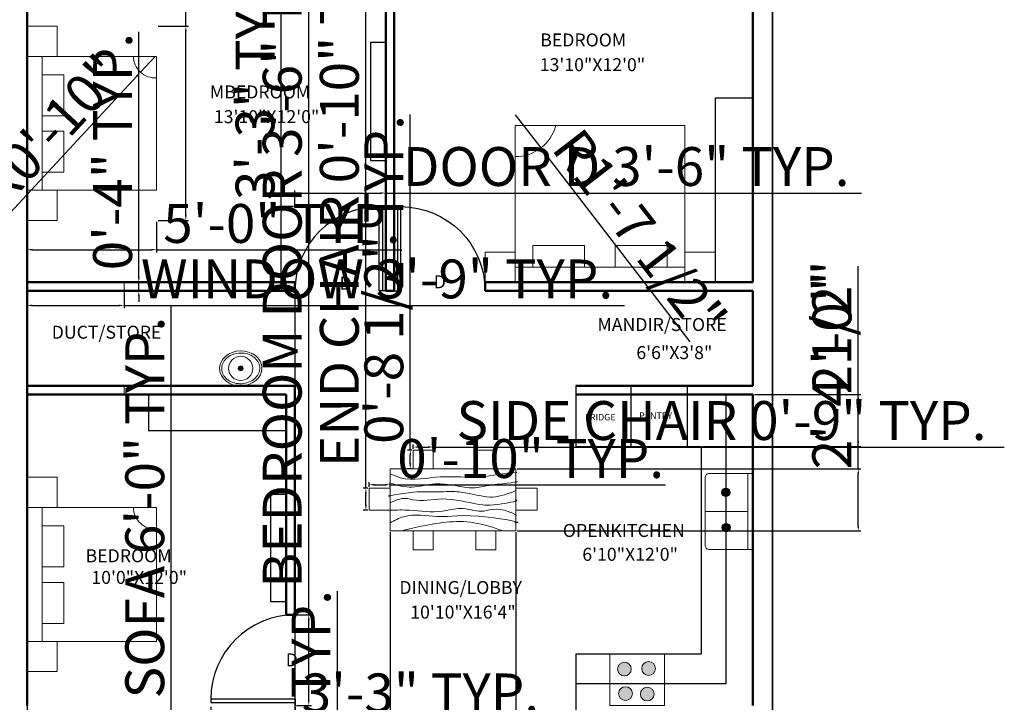
# Model space of a CAD drawing. Units: inches. Extents: x 2040 to 2729, y 1653 to 2621.
# Tile 3 of 4: x 2273 to 2729, y 1979 to 2295. Entities that reach past the tile are written whole.
import ezdxf

# ---------------------------------------------------------------- set-up
doc = ezdxf.new("R2010")
doc.units = ezdxf.units.IN
doc.layers.get('0').update_dxf_attribs({"color": 111})
for name, color, linetype, lineweight in [('A-ANNO-DIMS', 10, 'Continuous', 18), ('A-ANNO-TEXT', 30, 'Continuous', 18), ('A-AREA-IDEN', 6, 'Continuous', 18), ('A-DOOR', 50, 'Continuous', 25), ('A-EQPM', 8, 'Continuous', 18), ('A-FIXT-PATT', 18, 'Continuous', 13), ('A-FLOR-CASE', 30, 'Continuous', 25), ('A-FLOR-FIXT', 4, 'Continuous', 18), ('A-FURN', 30, 'Continuous', 18), ('A-GLAZ', 31, 'Continuous', 18), ('A-WALL', 7, 'Continuous', 50), ('C-PROP', 111, 'Continuous', 35)]:
    doc.layers.add(name, color=color, linetype=linetype, lineweight=lineweight)
doc.styles.get("Standard").update_dxf_attribs({"font": 'arial.ttf'})
doc.dimstyles.new('ISO-25', dxfattribs={"dimtxt": 18, "dimasz": 2.5, "dimexe": 1.25, "dimexo": 0.625, "dimtad": 1, "dimdec": 0, "dimlunit": 3, "dimtxsty": 'Standard', "dimcen": 2.5, "dimadec": 0, "dimazin": 0, "dimtfac": 1, "dimtdec": 0, "dimtmove": 0, "dimatfit": 3, "dimfxl": 1, "dimarcsym": 0})

# ---------------------------------------------------------------- blocks, each defined once
blk = doc.blocks.new('BASIN-OVAL')
h = blk.add_hatch(color=256)
h.dxf.hatch_style = 1
h.paths.add_polyline_path([(1.14, 0, 1), (-1.14, 0, 1)])
for radius in [5.58, 1.14]:
    blk.add_circle((0, 0), radius)
blk.add_ellipse((0, 0), major_axis=(9.81, 0.23), ratio=0.826688)
blk.add_open_spline([(8.81, 0.21), (8.8, 0.81), (8.69, 1.4), (8.2, 2.81), (7.72, 3.6), (6.41, 5.01), (5.59, 5.62), (3.7, 6.55), (2.64, 6.87), (0.44, 7.17), (-0.7, 7.15), (-2.89, 6.76), (-3.94, 6.39), (-5.79, 5.39), (-6.59, 4.75), (-7.85, 3.29), (-8.3, 2.48), (-8.82, 0.79), (-8.88, -0.08), (-8.62, -1.78), (-8.3, -2.62), (-7.28, -4.16), (-6.59, -4.86), (-4.92, -6.01), (-3.94, -6.46), (-1.83, -7.03), (-0.7, -7.16), (1.53, -7.05), (2.64, -6.83), (4.67, -6.06), (5.59, -5.52), (7.11, -4.23), (7.72, -3.47), (8.55, -1.86), (8.78, -1), (8.82, -0.02), (8.82, 0.09), (8.81, 0.21)], degree=3, knots=[0, 0, 0, 0, 0.259704, 0.259704, 0.633026, 0.633026, 1.006347, 1.006347, 1.379668, 1.379668, 1.752989, 1.752989, 2.12631, 2.12631, 2.499631, 2.499631, 2.872952, 2.872952, 3.246274, 3.246274, 3.619595, 3.619595, 3.992916, 3.992916, 4.366237, 4.366237, 4.739558, 4.739558, 5.112879, 5.112879, 5.486201, 5.486201, 5.859522, 5.859522, 6.232843, 6.232843, 6.283185, 6.283185, 6.283185, 6.283185])
blk = doc.blocks.new('BED-WITH-NIGHTSTANDS')
blk.add_line((7, 0), (7, -62))
for points in [[(0, 0), (14, 0), (14, 14), (0, 14)], [(0, 0), (60, 0), (60, -62), (0, -62)], [(7, -8.54), (17, -8.54), (17, -27.54), (7, -27.54)], [(7, -53.68), (17, -53.68), (17, -34.68), (7, -34.68)], [(0, -62), (14, -62), (14, -76), (0, -76)]]:
    blk.add_lwpolyline(points, close=True)
blk.add_arc((59.24, 0), 9.97, 180, 274.3506)
blk = doc.blocks.new('DOOR-39IN')
for p, q in [((0, 0), (0, 39)), ((0, 39), (1.5, 39)), ((1.5, 39), (1.5, 0)), ((3, 0), (0, 0))]:
    blk.add_line(p, q)
blk.add_arc((0, 0), 39, 90, 180)
blk = doc.blocks.new('DOOR-39IN-ALT')
for p, q in [((0, 0), (-39, 0)), ((-39, 0), (-39, -1.5)), ((0, 0), (0, -3)), ((0, -3), (0, 0)), ((-39, -1.5), (0, -1.5)), ((-39, -1.5), (0, -1.5))]:
    blk.add_line(p, q)
blk.add_arc((0, 0), 39, 90, 180)
blk = doc.blocks.new('WINDOW-45IN')
blk.add_lwpolyline([(0, 0), (45, 0), (45, -4), (0, -4)], close=True)
blk = doc.blocks.new('DINING-CHAIR-SIDE')
blk.add_lwpolyline([(0, 0), (9.24, 0), (9.24, 8.72), (0, 8.72)], close=True)
blk = doc.blocks.new('DINING-CHAIR-END')
blk.add_lwpolyline([(0, 0), (-9.76, 0), (-9.76, -10.23), (0, -10.23)], close=True)
blk = doc.blocks.new('*D21')
at = {"layer": 'A-ANNO-DIMS', "color": 0, "lineweight": -2, "transparency": 16777216}
for p, q in [((2455.26, 2096.6), (2455.26, 2098.61)), ((2457.76, 2097.36), (2462.01, 2097.36)), ((2464.51, 2096.6), (2464.51, 2098.61)), ((2464.51, 2097.36), (2728.79, 2097.36))]:
    blk.add_line(p, q, dxfattribs=at)
at = {"layer": 'A-ANNO-DIMS', "color": 0, "transparency": 16777216}
for points in [[(2457.76, 2097.77), (2457.76, 2096.94), (2455.26, 2097.36)], [(2462.01, 2097.77), (2462.01, 2096.94), (2464.51, 2097.36)]]:
    blk.add_solid(points, dxfattribs=at)
at = {"layer": 'Defpoints', "color": 0, "transparency": 16777216}
for p in [(2464.51, 2097.36), (2455.26, 2095.97), (2464.51, 2095.97)]:
    blk.add_point(p, dxfattribs=at)
at = {"layer": 'A-ANNO-DIMS', "color": 0, "transparency": 16777216, "insert": (2597.9, 2107.29), "char_height": 18, "attachment_point": 5}
blk.add_mtext('SIDE CHAIR 0\'-9" TYP.', dxfattribs=at)
blk = doc.blocks.new('*D22')
at = {"layer": 'A-ANNO-DIMS', "color": 0, "lineweight": -2, "transparency": 16777216}
for p, q in [((2453.88, 2095.97), (2453.88, 2251.38)), ((2454.64, 2095.97), (2452.63, 2095.97)), ((2453.88, 2089.75), (2453.88, 2093.47)), ((2454.64, 2087.25), (2452.63, 2087.25))]:
    blk.add_line(p, q, dxfattribs=at)
at = {"layer": 'A-ANNO-DIMS', "color": 0, "transparency": 16777216}
for points in [[(2453.46, 2093.47), (2454.29, 2093.47), (2453.88, 2095.97)], [(2453.46, 2089.75), (2454.29, 2089.75), (2453.88, 2087.25)]]:
    blk.add_solid(points, dxfattribs=at)
at = {"layer": 'Defpoints', "color": 0, "transparency": 16777216}
for p in [(2453.88, 2095.97), (2455.26, 2095.97), (2455.26, 2087.25)]:
    blk.add_point(p, dxfattribs=at)
at = {"layer": 'A-ANNO-DIMS', "color": 0, "transparency": 16777216, "insert": (2443.94, 2174.93), "char_height": 18, "attachment_point": 5, "rotation": 90}
blk.add_mtext('0\'-8 1/2" TYP.', dxfattribs=at)
blk = doc.blocks.new('*D24')
at = {"layer": 'A-ANNO-DIMS', "color": 0, "lineweight": -2, "transparency": 16777216}
for p, q in [((2420.15, 1876.92), (2420.15, 2030.64)), ((2423.85, 1876.92), (2418.9, 1876.92)), ((2420.15, 1861.83), (2420.15, 1874.42)), ((2423.85, 1859.33), (2418.9, 1859.33))]:
    blk.add_line(p, q, dxfattribs=at)
at = {"layer": 'A-ANNO-DIMS', "color": 0, "transparency": 16777216}
for points in [[(2419.73, 1874.42), (2420.57, 1874.42), (2420.15, 1876.92)], [(2419.73, 1861.83), (2420.57, 1861.83), (2420.15, 1859.33)]]:
    blk.add_solid(points, dxfattribs=at)
at = {"layer": 'Defpoints', "color": 0, "transparency": 16777216}
for p in [(2420.15, 1876.92), (2424.47, 1876.92), (2424.47, 1859.33)]:
    blk.add_point(p, dxfattribs=at)
at = {"layer": 'A-ANNO-DIMS', "color": 0, "transparency": 16777216, "insert": (2410.22, 1955.03), "char_height": 18, "attachment_point": 5, "rotation": 90}
blk.add_mtext('1\'-5 1/2" TYP.', dxfattribs=at)
blk = doc.blocks.new('*D25')
at = {"layer": 'A-ANNO-DIMS', "color": 0, "lineweight": -2, "transparency": 16777216}
for p, q in [((2400.47, 2209.29), (2400.47, 2216.21)), ((2402.97, 2214.96), (2439.97, 2214.96)), ((2442.47, 2209.29), (2442.47, 2216.21)), ((2442.47, 2214.96), (2662.62, 2214.96))]:
    blk.add_line(p, q, dxfattribs=at)
at = {"layer": 'A-ANNO-DIMS', "color": 0, "transparency": 16777216}
for points in [[(2402.97, 2215.38), (2402.97, 2214.54), (2400.47, 2214.96)], [(2439.97, 2215.38), (2439.97, 2214.54), (2442.47, 2214.96)]]:
    blk.add_solid(points, dxfattribs=at)
at = {"layer": 'Defpoints', "color": 0, "transparency": 16777216}
for p in [(2442.47, 2214.96), (2400.47, 2208.66), (2442.47, 2208.66)]:
    blk.add_point(p, dxfattribs=at)
at = {"layer": 'A-ANNO-DIMS', "color": 0, "transparency": 16777216, "insert": (2553.8, 2224.91), "char_height": 18, "attachment_point": 5}
blk.add_mtext('DOOR D 3\'-6" TYP.', dxfattribs=at)
blk = doc.blocks.new('*D26')
at = {"layer": 'A-ANNO-DIMS', "color": 0, "lineweight": -2, "transparency": 16777216}
for p, q in [((2394.17, 2208.66), (2394.17, 2322.12)), ((2399.85, 2208.66), (2392.92, 2208.66)), ((2394.17, 2172.16), (2394.17, 2206.16)), ((2399.85, 2169.66), (2392.92, 2169.66))]:
    blk.add_line(p, q, dxfattribs=at)
at = {"layer": 'A-ANNO-DIMS', "color": 0, "transparency": 16777216}
for points in [[(2393.76, 2206.16), (2394.59, 2206.16), (2394.17, 2208.66)], [(2393.76, 2172.16), (2394.59, 2172.16), (2394.17, 2169.66)]]:
    blk.add_solid(points, dxfattribs=at)
at = {"layer": 'Defpoints', "color": 0, "transparency": 16777216}
for p in [(2394.17, 2208.66), (2400.47, 2208.66), (2400.47, 2169.66)]:
    blk.add_point(p, dxfattribs=at)
at = {"layer": 'A-ANNO-DIMS', "color": 0, "transparency": 16777216, "insert": (2384.35, 2266.64), "char_height": 18, "attachment_point": 5, "rotation": 90}
blk.add_mtext('3\'-3" TYP.', dxfattribs=at)
blk = doc.blocks.new('*D27')
at = {"layer": 'A-ANNO-DIMS', "color": 0, "lineweight": -2, "transparency": 16777216}
for p, q in [((2349.97, 2292.24), (2349.97, 2606.15)), ((2337.1, 2292.24), (2351.22, 2292.24)), ((2349.97, 2204.74), (2349.97, 2289.74)), ((2337.1, 2202.24), (2351.22, 2202.24))]:
    blk.add_line(p, q, dxfattribs=at)
at = {"layer": 'A-ANNO-DIMS', "color": 0, "transparency": 16777216}
for points in [[(2349.56, 2289.74), (2350.39, 2289.74), (2349.97, 2292.24)], [(2349.56, 2204.74), (2350.39, 2204.74), (2349.97, 2202.24)]]:
    blk.add_solid(points, dxfattribs=at)
at = {"layer": 'Defpoints', "color": 0, "transparency": 16777216}
for p in [(2336.47, 2292.24), (2349.97, 2292.24), (2336.47, 2202.24)]:
    blk.add_point(p, dxfattribs=at)
at = {"layer": 'A-ANNO-DIMS', "color": 0, "transparency": 16777216, "insert": (2340.04, 2450.44), "char_height": 18, "attachment_point": 5, "rotation": 90}
blk.add_mtext('BED ASSEMBLY 7\'-6" TYP.', dxfattribs=at)
blk = doc.blocks.new('*D28')
at = {"layer": 'A-ANNO-DIMS', "color": 0, "lineweight": -2, "transparency": 16777216}
for p, q in [((2276.47, 2201.61), (2276.47, 2187.49)), ((2336.47, 2201.61), (2336.47, 2187.49)), ((2278.97, 2188.74), (2333.97, 2188.74)), ((2336.47, 2188.74), (2449.94, 2188.74))]:
    blk.add_line(p, q, dxfattribs=at)
at = {"layer": 'A-ANNO-DIMS', "color": 0, "transparency": 16777216}
for points in [[(2278.97, 2189.15), (2278.97, 2188.32), (2276.47, 2188.74)], [(2333.97, 2189.15), (2333.97, 2188.32), (2336.47, 2188.74)]]:
    blk.add_solid(points, dxfattribs=at)
at = {"layer": 'Defpoints', "color": 0, "transparency": 16777216}
for p in [(2276.47, 2202.24), (2336.47, 2202.24), (2336.47, 2188.74)]:
    blk.add_point(p, dxfattribs=at)
at = {"layer": 'A-ANNO-DIMS', "color": 0, "transparency": 16777216, "insert": (2394.46, 2198.55), "char_height": 18, "attachment_point": 5}
blk.add_mtext('5\'-0" TYP.', dxfattribs=at)
blk = doc.blocks.new('*D29')
at = {"layer": 'A-ANNO-DIMS', "color": 0, "lineweight": -2, "transparency": 16777216}
for p, q in [((2343.24, 1973.66), (2343.24, 2162.49)), ((2333.07, 1973.66), (2344.49, 1973.66)), ((2343.24, 1904.16), (2343.24, 1971.16)), ((2333.07, 1901.66), (2344.49, 1901.66))]:
    blk.add_line(p, q, dxfattribs=at)
at = {"layer": 'A-ANNO-DIMS', "color": 0, "transparency": 16777216}
for points in [[(2342.83, 1971.16), (2343.66, 1971.16), (2343.24, 1973.66)], [(2342.83, 1904.16), (2343.66, 1904.16), (2343.24, 1901.66)]]:
    blk.add_solid(points, dxfattribs=at)
at = {"layer": 'Defpoints', "color": 0, "transparency": 16777216}
for p in [(2332.44, 1973.66), (2343.24, 1973.66), (2332.44, 1901.66)]:
    blk.add_point(p, dxfattribs=at)
at = {"layer": 'A-ANNO-DIMS', "color": 0, "transparency": 16777216, "insert": (2333.3, 2069.33), "char_height": 18, "attachment_point": 5, "rotation": 90}
blk.add_mtext('SOFA 6\'-0" TYP.', dxfattribs=at)
blk = doc.blocks.new('*D33')
at = {"layer": 'A-ANNO-DIMS', "color": 0, "lineweight": -2, "transparency": 16777216}
for p, q in [((2406.86, 2019.66), (2406.86, 2351.67)), ((2401.19, 2019.66), (2408.11, 2019.66)), ((2406.86, 1980.16), (2406.86, 2017.16)), ((2401.19, 1977.66), (2408.11, 1977.66))]:
    blk.add_line(p, q, dxfattribs=at)
at = {"layer": 'A-ANNO-DIMS', "color": 0, "transparency": 16777216}
for points in [[(2406.45, 2017.16), (2407.28, 2017.16), (2406.86, 2019.66)], [(2406.45, 1980.16), (2407.28, 1980.16), (2406.86, 1977.66)]]:
    blk.add_solid(points, dxfattribs=at)
at = {"layer": 'Defpoints', "color": 0, "transparency": 16777216}
for p in [(2400.56, 2019.66), (2406.86, 2019.66), (2400.56, 1977.66)]:
    blk.add_point(p, dxfattribs=at)
at = {"layer": 'A-ANNO-DIMS', "color": 0, "transparency": 16777216, "insert": (2396.92, 2186.92), "char_height": 18, "attachment_point": 5, "rotation": 90}
blk.add_mtext('BEDROOM DOOR 3\'-6" TYP.', dxfattribs=at)
blk = doc.blocks.new('*D34')
at = {"layer": 'A-ANNO-DIMS', "color": 0, "lineweight": -2, "transparency": 16777216}
for p, q in [((2361.56, 1977.04), (2361.56, 1970.11)), ((2400.56, 1977.04), (2400.56, 1970.11)), ((2364.06, 1971.36), (2398.06, 1971.36)), ((2400.56, 1971.36), (2514.02, 1971.36))]:
    blk.add_line(p, q, dxfattribs=at)
at = {"layer": 'A-ANNO-DIMS', "color": 0, "transparency": 16777216}
for points in [[(2364.06, 1971.78), (2364.06, 1970.94), (2361.56, 1971.36)], [(2398.06, 1971.78), (2398.06, 1970.94), (2400.56, 1971.36)]]:
    blk.add_solid(points, dxfattribs=at)
at = {"layer": 'Defpoints', "color": 0, "transparency": 16777216}
for p in [(2361.56, 1977.66), (2400.56, 1977.66), (2400.56, 1971.36)]:
    blk.add_point(p, dxfattribs=at)
at = {"layer": 'A-ANNO-DIMS', "color": 0, "transparency": 16777216, "insert": (2458.54, 1981.18), "char_height": 18, "attachment_point": 5}
blk.add_mtext('3\'-3" TYP.', dxfattribs=at)
blk = doc.blocks.new('*D35')
at = {"layer": 'A-ANNO-DIMS', "color": 0, "lineweight": -2, "transparency": 16777216}
for p, q in [((2276.47, 2169.04), (2276.47, 2161.66)), ((2321.47, 2169.04), (2321.47, 2161.66)), ((2278.97, 2162.91), (2318.97, 2162.91)), ((2321.47, 2162.91), (2553, 2162.91))]:
    blk.add_line(p, q, dxfattribs=at)
at = {"layer": 'A-ANNO-DIMS', "color": 0, "transparency": 16777216}
for points in [[(2278.97, 2163.33), (2278.97, 2162.49), (2276.47, 2162.91)], [(2318.97, 2163.33), (2318.97, 2162.49), (2321.47, 2162.91)]]:
    blk.add_solid(points, dxfattribs=at)
at = {"layer": 'Defpoints', "color": 0, "transparency": 16777216}
for p in [(2276.47, 2169.66), (2321.47, 2169.66), (2321.47, 2162.91)]:
    blk.add_point(p, dxfattribs=at)
at = {"layer": 'A-ANNO-DIMS', "color": 0, "transparency": 16777216, "insert": (2438.49, 2172.86), "char_height": 18, "attachment_point": 5}
blk.add_mtext('WINDOW 3\'-9" TYP.', dxfattribs=at)
blk = doc.blocks.new('*D36')
at = {"layer": 'A-ANNO-DIMS', "color": 0, "lineweight": -2, "transparency": 16777216}
for p, q in [((2328.22, 2176.16), (2328.22, 2289.63)), ((2322.1, 2173.66), (2329.47, 2173.66)), ((2322.1, 2169.66), (2329.47, 2169.66)), ((2328.22, 2169.66), (2328.22, 2173.66)), ((2328.22, 2167.16), (2328.22, 2164.66))]:
    blk.add_line(p, q, dxfattribs=at)
at = {"layer": 'A-ANNO-DIMS', "color": 0, "transparency": 16777216}
for points in [[(2327.81, 2176.16), (2328.64, 2176.16), (2328.22, 2173.66)], [(2327.81, 2167.16), (2328.64, 2167.16), (2328.22, 2169.66)]]:
    blk.add_solid(points, dxfattribs=at)
at = {"layer": 'Defpoints', "color": 0, "transparency": 16777216}
for p in [(2321.47, 2173.66), (2321.47, 2169.66), (2328.22, 2173.66)]:
    blk.add_point(p, dxfattribs=at)
at = {"layer": 'A-ANNO-DIMS', "color": 0, "transparency": 16777216, "insert": (2318.41, 2234.15), "char_height": 18, "attachment_point": 5, "rotation": 90}
blk.add_mtext('0\'-4" TYP.', dxfattribs=at)
blk = doc.blocks.new('*D39')
at = {"layer": 'A-ANNO-DIMS', "color": 0, "lineweight": -2, "transparency": 16777216}
for p, q in [((2433.3, 2078.37), (2433.3, 2350.18)), ((2434.21, 2078.37), (2432.05, 2078.37)), ((2433.3, 2070.64), (2433.3, 2075.87)), ((2434.21, 2068.14), (2432.05, 2068.14))]:
    blk.add_line(p, q, dxfattribs=at)
at = {"layer": 'A-ANNO-DIMS', "color": 0, "transparency": 16777216}
for points in [[(2432.88, 2075.87), (2433.72, 2075.87), (2433.3, 2078.37)], [(2432.88, 2070.64), (2433.72, 2070.64), (2433.3, 2068.14)]]:
    blk.add_solid(points, dxfattribs=at)
at = {"layer": 'Defpoints', "color": 0, "transparency": 16777216}
for p in [(2433.3, 2078.37), (2434.84, 2078.37), (2434.84, 2068.14)]:
    blk.add_point(p, dxfattribs=at)
at = {"layer": 'A-ANNO-DIMS', "color": 0, "transparency": 16777216, "insert": (2423.37, 2215.52), "char_height": 18, "attachment_point": 5, "rotation": 90}
blk.add_mtext('END CHAIR 0\'-10" TYP.', dxfattribs=at)
blk = doc.blocks.new('*D40')
at = {"layer": 'A-ANNO-DIMS', "color": 0, "lineweight": -2, "transparency": 16777216}
for p, q in [((2434.84, 2078.99), (2434.84, 2081.15)), ((2437.34, 2079.9), (2442.1, 2079.9)), ((2444.6, 2078.99), (2444.6, 2081.15)), ((2444.6, 2079.9), (2572.05, 2079.9))]:
    blk.add_line(p, q, dxfattribs=at)
at = {"layer": 'A-ANNO-DIMS', "color": 0, "transparency": 16777216}
for points in [[(2437.34, 2080.32), (2437.34, 2079.49), (2434.84, 2079.9)], [(2442.1, 2080.32), (2442.1, 2079.49), (2444.6, 2079.9)]]:
    blk.add_solid(points, dxfattribs=at)
at = {"layer": 'Defpoints', "color": 0, "transparency": 16777216}
for p in [(2434.84, 2078.37), (2444.6, 2079.9), (2444.6, 2078.37)]:
    blk.add_point(p, dxfattribs=at)
at = {"layer": 'A-ANNO-DIMS', "color": 0, "transparency": 16777216, "insert": (2509.57, 2089.72), "char_height": 18, "attachment_point": 5}
blk.add_mtext('0\'-10" TYP.', dxfattribs=at)
blk = doc.blocks.new('*D41')
at = {"layer": 'A-ANNO-DIMS', "color": 0, "lineweight": -2, "transparency": 16777216}
for p, q in [((2266.85, 2402.66), (2226.49, 2402.66)), ((2227.74, 1775.16), (2227.74, 2400.16)), ((2275.85, 1772.66), (2226.49, 1772.66))]:
    blk.add_line(p, q, dxfattribs=at)
at = {"layer": 'A-ANNO-DIMS', "color": 0, "transparency": 16777216}
for points in [[(2227.33, 2400.16), (2228.16, 2400.16), (2227.74, 2402.66)], [(2227.33, 1775.16), (2228.16, 1775.16), (2227.74, 1772.66)]]:
    blk.add_solid(points, dxfattribs=at)
at = {"layer": 'Defpoints', "color": 0, "transparency": 16777216}
for p in [(2227.74, 2402.66), (2267.47, 2402.66), (2276.47, 1772.66)]:
    blk.add_point(p, dxfattribs=at)
at = {"layer": 'A-ANNO-DIMS', "color": 0, "transparency": 16777216, "insert": (2217.93, 2087.66), "char_height": 18, "attachment_point": 5, "rotation": 90}
blk.add_mtext('52\'-6"', dxfattribs=at)
blk = doc.blocks.new('*D44')
at = {"layer": 'A-ANNO-DIMS', "color": 0, "lineweight": -2, "transparency": 16777216}
for p, q in [((2276.47, 2169.04), (2276.47, 1653.68)), ((2400.47, 2169.04), (2400.47, 1653.68)), ((2278.97, 1654.93), (2397.97, 1654.93))]:
    blk.add_line(p, q, dxfattribs=at)
at = {"layer": 'A-ANNO-DIMS', "color": 0, "transparency": 16777216}
for points in [[(2278.97, 1655.35), (2278.97, 1654.51), (2276.47, 1654.93)], [(2397.97, 1655.35), (2397.97, 1654.51), (2400.47, 1654.93)]]:
    blk.add_solid(points, dxfattribs=at)
at = {"layer": 'Defpoints', "color": 0, "transparency": 16777216}
for p in [(2276.47, 2169.66), (2400.47, 2169.66), (2400.47, 1654.93)]:
    blk.add_point(p, dxfattribs=at)
at = {"layer": 'A-ANNO-DIMS', "color": 0, "transparency": 16777216, "insert": (2338.47, 1664.75), "char_height": 18, "attachment_point": 5}
blk.add_mtext('10\'-4"', dxfattribs=at)
blk = doc.blocks.new('*D45')
at = {"layer": 'A-ANNO-DIMS', "color": 0, "lineweight": -2, "transparency": 16777216}
for p, q in [((2444.6, 2057.89), (2444.6, 1653.68)), ((2502.75, 2057.89), (2502.75, 1653.68)), ((2447.1, 1654.93), (2500.25, 1654.93)), ((2502.75, 1654.93), (2569.05, 1654.93))]:
    blk.add_line(p, q, dxfattribs=at)
at = {"layer": 'A-ANNO-DIMS', "color": 0, "transparency": 16777216}
for points in [[(2447.1, 1655.35), (2447.1, 1654.51), (2444.6, 1654.93)], [(2500.25, 1655.35), (2500.25, 1654.51), (2502.75, 1654.93)]]:
    blk.add_solid(points, dxfattribs=at)
at = {"layer": 'Defpoints', "color": 0, "transparency": 16777216}
for p in [(2444.6, 2058.52), (2502.75, 2058.52), (2502.75, 1654.93)]:
    blk.add_point(p, dxfattribs=at)
at = {"layer": 'A-ANNO-DIMS', "color": 0, "transparency": 16777216, "insert": (2537.15, 1664.75), "char_height": 18, "attachment_point": 5}
blk.add_mtext('4\'-10"', dxfattribs=at)
blk = doc.blocks.new('*D46')
at = {"layer": 'A-ANNO-DIMS', "color": 0, "lineweight": -2, "transparency": 16777216}
for p, q in [((2661.2, 2087.25), (2661.2, 2181.09)), ((2503.37, 2087.25), (2662.45, 2087.25)), ((2661.2, 2061.02), (2661.2, 2084.75)), ((2503.37, 2058.52), (2662.45, 2058.52))]:
    blk.add_line(p, q, dxfattribs=at)
at = {"layer": 'A-ANNO-DIMS', "color": 0, "transparency": 16777216}
for points in [[(2660.79, 2084.75), (2661.62, 2084.75), (2661.2, 2087.25)], [(2660.79, 2061.02), (2661.62, 2061.02), (2661.2, 2058.52)]]:
    blk.add_solid(points, dxfattribs=at)
at = {"layer": 'Defpoints', "color": 0, "transparency": 16777216}
for p in [(2502.75, 2087.25), (2661.2, 2087.25), (2502.75, 2058.52)]:
    blk.add_point(p, dxfattribs=at)
at = {"layer": 'A-ANNO-DIMS', "color": 0, "transparency": 16777216, "insert": (2651.27, 2135.42), "char_height": 18, "attachment_point": 5, "rotation": 90}
blk.add_mtext('2\'-4 1/2"', dxfattribs=at)
blk = doc.blocks.new('*D47')
at = {"layer": 'A-ANNO-DIMS', "color": 0, "lineweight": -2, "transparency": 16777216}
for p, q in [((2661.2, 2121.66), (2661.2, 2173.57)), ((2613.1, 2121.66), (2662.45, 2121.66)), ((2661.2, 2100.16), (2661.2, 2119.16)), ((2589.1, 2097.66), (2662.45, 2097.66))]:
    blk.add_line(p, q, dxfattribs=at)
at = {"layer": 'A-ANNO-DIMS', "color": 0, "transparency": 16777216}
for points in [[(2660.79, 2119.16), (2661.62, 2119.16), (2661.2, 2121.66)], [(2660.79, 2100.16), (2661.62, 2100.16), (2661.2, 2097.66)]]:
    blk.add_solid(points, dxfattribs=at)
at = {"layer": 'Defpoints', "color": 0, "transparency": 16777216}
for p in [(2612.47, 2121.66), (2661.2, 2121.66), (2588.47, 2097.66)]:
    blk.add_point(p, dxfattribs=at)
at = {"layer": 'A-ANNO-DIMS', "color": 0, "transparency": 16777216, "insert": (2651.39, 2148.86), "char_height": 18, "attachment_point": 5, "rotation": 90}
blk.add_mtext('2\'-0"', dxfattribs=at)
blk = doc.blocks.new('*D49')
at = {"layer": 'A-ANNO-DIMS', "color": 0, "lineweight": -2, "transparency": 16777216}
for p, q in [((2502.47, 2251.23), (2514.32, 2235.85)), ((2583.46, 2146.12), (2515.85, 2233.87))]:
    blk.add_line(p, q, dxfattribs=at)
at = {"layer": 'A-ANNO-DIMS', "color": 0, "transparency": 16777216}
blk.add_solid([(2516.18, 2234.12), (2515.52, 2233.61), (2514.32, 2235.85)], dxfattribs=at)
at = {"layer": 'Defpoints', "color": 0, "transparency": 16777216}
for p in [(2502.47, 2251.23), (2514.32, 2235.85)]:
    blk.add_point(p, dxfattribs=at)
at = {"layer": 'A-ANNO-DIMS', "color": 0, "transparency": 16777216, "insert": (2558.28, 2195.06), "char_height": 18, "attachment_point": 5, "rotation": 307.6136}
blk.add_mtext('R1\'-7 1/2"', dxfattribs=at)
blk = doc.blocks.new('*D50')
at = {"layer": 'A-ANNO-DIMS', "color": 0, "lineweight": -2, "transparency": 16777216}
for p, q in [((2335.72, 2278.24), (2328.94, 2270.92)), ((2244.45, 2179.76), (2327.24, 2269.09))]:
    blk.add_line(p, q, dxfattribs=at)
at = {"layer": 'A-ANNO-DIMS', "color": 0, "transparency": 16777216}
blk.add_solid([(2326.93, 2269.37), (2327.54, 2268.81), (2328.94, 2270.92)], dxfattribs=at)
at = {"layer": 'Defpoints', "color": 0, "transparency": 16777216}
for p in [(2335.72, 2278.24), (2328.94, 2270.92)]:
    blk.add_point(p, dxfattribs=at)
at = {"layer": 'A-ANNO-DIMS', "color": 0, "transparency": 16777216, "insert": (2277.8, 2230.18), "char_height": 18, "attachment_point": 5, "rotation": 47.1751}
blk.add_mtext('2X R0\'-10"', dxfattribs=at)

msp = doc.modelspace()

# ---------------------------------------------------------------- hatches: boundary and pattern name
at = {"layer": 'A-FIXT-PATT'}
h = msp.add_hatch(color=256, dxfattribs=at)
h.dxf.hatch_style = 1
h.paths.add_polyline_path([(2599.88, 2078.37, 0.414214), (2597.88, 2076.38, 0.414214), (2599.88, 2074.38)])
h = msp.add_hatch(color=256, dxfattribs=at)
h.dxf.hatch_style = 1
h.paths.add_polyline_path([(2599.88, 2078.37), (2599.88, 2074.38, 0.414214), (2601.87, 2076.38, 0.414214)])
h = msp.add_hatch(color=256, dxfattribs=at)
h.dxf.hatch_style = 1
h.paths.add_polyline_path([(2599.88, 2062.02, 0.390218), (2598.05, 2060.04, 0.390218), (2599.88, 2058.05)])
h = msp.add_hatch(color=256, dxfattribs=at)
h.dxf.hatch_style = 1
h.paths.add_polyline_path([(2599.88, 2062.02), (2599.88, 2058.05, 0.438623), (2602.04, 2060.04, 0.438623)])
h = msp.add_hatch(color=256, dxfattribs=at)
h.dxf.hatch_style = 1
h.paths.add_polyline_path([(2549.76, 1994.57, 1), (2556.13, 1994.57, 1)])
h = msp.add_hatch(color=256, dxfattribs=at)
h.dxf.hatch_style = 1
h.paths.add_polyline_path([(2560.98, 1994.82, 1), (2567.36, 1994.82, 1)])
h = msp.add_hatch(color=256, dxfattribs=at)
h.dxf.hatch_style = 1
h.paths.add_polyline_path([(2550.26, 1983.22, 1), (2556.64, 1983.22, 1)])
h = msp.add_hatch(color=256, dxfattribs=at)
h.dxf.hatch_style = 1
h.paths.add_polyline_path([(2560.34, 1982.97, 1), (2566.72, 1982.97, 1)])

# ---------------------------------------------------------------- linework, layer by layer
at = {"layer": 'A-EQPM'}
msp.add_lwpolyline([(2571.47, 1977.66), (2546.15, 1977.66), (2546.15, 2001.66), (2571.47, 2001.66)], close=True, dxfattribs=at)
for centre in [(2552.94, 1994.57), (2564.17, 1994.82), (2553.45, 1983.22), (2563.53, 1982.97)]:
    msp.add_circle(centre, 3.19, dxfattribs=at)
at = {"layer": 'A-FLOR-CASE'}
for p, q in [((2595, 2258.97), (2612.47, 2258.97)), ((2595, 2258.97), (2595, 2173.66)), ((2530.47, 2125.66), (2530.47, 2097.66)), ((2556.01, 2125.66), (2556.01, 2097.66)), ((2582.01, 2125.66), (2582.01, 2097.66)), ((2332.65, 2121.66), (2332.65, 2104.96)), ((2599.88, 2121.66), (2599.88, 1987.66)), ((2332.65, 2104.96), (2396.47, 2104.96)), ((2530.47, 2097.66), (2588.47, 2097.66)), ((2588.47, 2097.66), (2588.47, 2001.66)), ((2530.47, 2001.66), (2588.47, 2001.66)), ((2530.47, 2001.66), (2530.47, 1973.66)), ((2599.88, 1987.66), (2530.47, 1987.66))]:
    msp.add_line(p, q, dxfattribs=at)
for points in [[(2442.47, 2284.65), (2435.5, 2284.65), (2435.5, 2230.03), (2442.47, 2230.03)], [(2396.47, 2025.68), (2389.28, 2025.68), (2389.28, 2075.47), (2396.47, 2075.47)]]:
    msp.add_lwpolyline(points, close=True, dxfattribs=at)
at = {"layer": 'A-FLOR-FIXT'}
for p, q in [((2610.01, 2085.08), (2610.01, 2049.93)), ((2590.29, 2067.5), (2610.01, 2067.5))]:
    msp.add_line(p, q, dxfattribs=at)
msp.add_lwpolyline([(2612.47, 2085.08), (2592.29, 2085.08, 0.414214), (2590.29, 2083.08), (2590.29, 2051.93, 0.414214), (2592.29, 2049.93), (2612.47, 2049.93)], format="xyb", close=True, dxfattribs=at)
for centre in [(2599.88, 2076.38), (2600.04, 2060.04)]:
    msp.add_circle(centre, 1.99, dxfattribs=at)
at = {"layer": 'A-FURN'}
msp.add_line((2502.47, 2180.66), (2581, 2180.66), dxfattribs=at)
for points in [[(2581, 2173.66), (2502.47, 2173.66), (2502.47, 2246.28), (2581, 2246.28)], [(2488.47, 2173.66), (2502.47, 2173.66), (2502.47, 2187.66), (2488.47, 2187.66)], [(2510.51, 2180.66), (2534.51, 2180.66), (2534.51, 2190.66), (2510.51, 2190.66)], [(2572.71, 2180.66), (2548.71, 2180.66), (2548.71, 2190.66), (2572.71, 2190.66)], [(2595, 2173.66), (2581, 2173.66), (2581, 2187.66), (2595, 2187.66)], [(2444.6, 2087.25), (2502.75, 2087.25), (2502.75, 2058.52), (2444.6, 2058.52)]]:
    msp.add_lwpolyline(points, close=True, dxfattribs=at)
msp.add_arc((2502.47, 2251.23), 19.42, 270, 345.2278, dxfattribs=at)
for points, knots in [([(2444.6, 2084.96), (2446.13, 2084.28), (2453.41, 2081.02), (2468.02, 2084.82), (2485.79, 2082.26), (2497.42, 2085.53), (2503, 2085.51), (2503.13, 2085.51)], [0, 0, 0, 0, 4.987596, 23.666071, 42.261233, 58.618164, 58.998049, 58.998049, 58.998049, 58.998049]), ([(2444.6, 2080.61), (2447.98, 2079.66), (2454.88, 2077.73), (2467.35, 2082.05), (2481.47, 2077.22), (2489.92, 2079.99), (2506.42, 2081.33), (2502.53, 2081.32), (2502.41, 2081.32)], [0, 0, 0, 0, 10.26646, 20.975536, 38.714611, 47.756573, 58.716362, 59.048634, 59.048634, 59.048634, 59.048634]), ([(2502.75, 2077.21), (2499.21, 2075.79), (2492.18, 2072.95), (2482.22, 2075.93), (2473.6, 2077), (2464.15, 2076.32), (2458.19, 2077.24), (2440.98, 2074.52), (2444.63, 2074.52), (2444.65, 2074.52)], [0, 0, 0, 0, 11.111976, 22.078966, 29.803528, 37.797066, 48.084955, 58.910579, 58.965396, 58.965396, 58.965396, 58.965396]), ([(2444.6, 2071.52), (2446.97, 2072.64), (2450.4, 2074.26), (2458.4, 2071.77), (2469.3, 2074.78), (2484.7, 2070.59), (2491.68, 2070.03), (2505, 2072.58), (2502.48, 2072.92), (2502.34, 2072.94)], [0, 0, 0, 0, 7.464989, 10.770346, 24.386161, 40.948091, 52.18542, 58.944004, 59.359914, 59.359914, 59.359914, 59.359914]), ([(2444.6, 2068.14), (2447.56, 2068.21), (2455.59, 2068.42), (2466.63, 2066.42), (2477.3, 2069.96), (2488.76, 2065.94), (2493.27, 2070.59), (2503.83, 2065.58), (2502.68, 2065.59), (2502.65, 2065.59)], [0, 0, 0, 0, 8.917191, 24.117795, 32.67851, 42.179381, 55.557912, 58.800504, 58.89539, 58.89539, 58.89539, 58.89539]), ([(2444.6, 2062.27), (2446.61, 2063.38), (2453.09, 2066.97), (2470.59, 2063.77), (2479.2, 2067.38), (2507.17, 2062.24), (2502.38, 2062.27), (2502.18, 2062.27)], [0, 0, 0, 0, 6.846542, 22.03938, 45.858195, 59.048704, 59.618361, 59.618361, 59.618361, 59.618361]), ([(2449.52, 2058.52), (2452.17, 2059.15), (2463.17, 2061.77), (2479.68, 2064.46), (2492.41, 2060.07), (2496.91, 2058.52)], [0, 0, 0, 0, 8.18394, 34.056627, 48.201517, 48.201517, 48.201517, 48.201517])]:
    msp.add_open_spline(points, degree=3, knots=knots, dxfattribs=at)
at = {"layer": 'A-WALL'}
for p, q in [((2276.47, 1977.66), (2276.47, 2393.66)), ((2446.47, 2169.66), (2446.47, 2393.66)), ((2612.47, 2393.66), (2612.47, 2173.66)), ((2442.47, 2169.66), (2442.47, 2317.66)), ((2276.47, 2173.66), (2400.47, 2173.66)), ((2276.47, 2169.66), (2400.47, 2169.66)), ((2400.47, 2169.66), (2400.47, 2173.66)), ((2442.47, 2169.66), (2446.47, 2169.66)), ((2488.47, 2173.66), (2612.47, 2173.66)), ((2488.47, 2169.66), (2488.47, 2173.66)), ((2488.47, 2169.66), (2612.47, 2169.66)), ((2612.47, 2169.66), (2612.47, 2125.66)), ((2276.47, 2125.66), (2400.47, 2125.66)), ((2400.47, 2019.66), (2400.47, 2125.66)), ((2530.47, 2125.66), (2612.47, 2125.66)), ((2276.47, 2121.66), (2396.47, 2121.66)), ((2396.47, 2019.66), (2396.47, 2121.66)), ((2530.47, 2121.66), (2612.47, 2121.66)), ((2612.47, 2121.66), (2612.47, 1977.66)), ((2396.47, 2019.66), (2400.47, 2019.66))]:
    msp.add_line(p, q, dxfattribs=at)
at = {"layer": 'C-PROP'}
msp.add_lwpolyline([(2267.47, 2402.66), (2621.47, 2402.66), (2621.47, 1694.66), (2267.47, 1694.66)], close=True, dxfattribs=at)

# ---------------------------------------------------------------- block references
at = {"layer": 'A-DOOR'}
for name, p in [('DOOR-39IN', (2439.47, 2169.66)), ('DOOR-39IN-ALT', (2400.56, 1980.66))]:
    msp.add_blockref(name, p, dxfattribs=at)
at = {"layer": 'A-DOOR', "extrusion": (0, 0, -1), "zscale": -1}
msp.add_blockref('DOOR-39IN', (-2449.47, 2169.66), dxfattribs=at)
at = {"layer": 'A-FLOR-FIXT'}
msp.add_blockref('BASIN-OVAL', (2375.38, 2133.78), dxfattribs=at)
at = {"layer": 'A-FURN'}
for name, p in [('BED-WITH-NIGHTSTANDS', (2276.47, 2278.24)), ('DINING-CHAIR-SIDE', (2455.26, 2087.25)), ('DINING-CHAIR-SIDE', (2484.18, 2087.25)), ('BED-WITH-NIGHTSTANDS', (2276.47, 2069.36)), ('DINING-CHAIR-END', (2444.6, 2078.37))]:
    msp.add_blockref(name, p, dxfattribs=at)
at = {"layer": 'A-FURN', "extrusion": (0, 0, -1), "zscale": -1}
msp.add_blockref('DINING-CHAIR-END', (-2502.75, 2078.37), dxfattribs=at)
at = {"layer": 'A-FURN', "extrusion": (0, 0, -1), "zscale": -1, "rotation": 180}
for p in [(-2455.26, 2058.52), (-2484.18, 2058.52)]:
    msp.add_blockref('DINING-CHAIR-SIDE', p, dxfattribs=at)
at = {"layer": 'A-GLAZ'}
for p in [(2276.47, 2173.66), (2276.47, 2125.66)]:
    msp.add_blockref('WINDOW-45IN', p, dxfattribs=at)

# ---------------------------------------------------------------- texts
at = {"layer": 'A-ANNO-TEXT'}
for tag, p, height in [('D', (2421.08, 2170.22), 6), ('D', (2464.72, 2170.86), 6), ('FRIDGE', (2534.74, 2109.7), 3), ('PANTRY', (2559.78, 2110.37), 3), ('D', (2396.22, 1995.81), 6)]:
    msp.add_attdef(tag, p, '', height=height, dxfattribs=at)
at = {"layer": 'A-AREA-IDEN'}
for tag, p in [('BEDROOM', (2513.99, 2282.84)), ('13\'10"X12\'0"', (2513.78, 2271.4)), ('MBEDROOM', (2361.09, 2258.76)), ('13\'10"X12\'0"', (2362.97, 2247.33)), ('MANDIR/STORE', (2540.47, 2151.09)), ('DUCT/STORE', (2287.92, 2147.53)), ('6\'6"X3\'8"', (2558.49, 2138.09)), ('OPENKITCHEN', (2524.45, 2055.72)), ('6\'10"X12\'0"', (2533.48, 2044.69)), ('BEDROOM', (2303.58, 2044.02)), ('10\'0"X12\'0"', (2306.26, 2033.99)), ('DINING/LOBBY', (2448.82, 2029.31)), ('10\'10"X16\'4"', (2453.84, 2017.94))]:
    msp.add_attdef(tag, p, '', height=6, dxfattribs=at)

# ---------------------------------------------------------------- dimensions: what is measured, and where the dimension line sits
at = {"layer": 'A-ANNO-DIMS'}
for base, p1, p2, text, picture, middle in [((2349.97, 2292.24), (2336.47, 2202.24), (2336.47, 2292.24), 'BED ASSEMBLY <> TYP.', '*D27', (2340.04, 2450.44)), ((2406.86, 2019.66), (2400.56, 1977.66), (2400.56, 2019.66), 'BEDROOM DOOR <> TYP.', '*D33', (2396.92, 2186.92)), ((2433.3, 2078.37), (2434.84, 2068.14), (2434.84, 2078.37), 'END CHAIR <> TYP.', '*D39', (2423.37, 2215.52)), ((2394.17, 2208.66), (2400.47, 2169.66), (2400.47, 2208.66), '<> TYP.', '*D26', (2384.35, 2266.64)), ((2328.22, 2173.66), (2321.47, 2169.66), (2321.47, 2173.66), '<> TYP.', '*D36', (2318.41, 2234.15)), ((2453.88, 2095.97), (2455.26, 2087.25), (2455.26, 2095.97), '<> TYP.', '*D22', (2443.94, 2174.93)), ((2343.24, 1973.66), (2332.44, 1901.66), (2332.44, 1973.66), 'SOFA <> TYP.', '*D29', (2333.3, 2069.33)), ((2420.15, 1876.92), (2424.47, 1859.33), (2424.47, 1876.92), '<> TYP.', '*D24', (2410.22, 1955.03))]:
    dim = msp.add_linear_dim(base=base, p1=p1, p2=p2, angle=90, text=text, dimstyle='ISO-25', override={"dimdec": 1, "dimlfac": 1, "dimrnd": 0, "dimzin": 1, "dimdsep": 46, "dimlunit": 4, "dimfrac": 2}, dxfattribs=at)
    dim.commit()
    dim.dimension.update_dxf_attribs({"geometry": picture, "text_midpoint": middle})
for base, p1, p2, picture, middle in [((2227.74, 2402.66), (2276.47, 1772.66), (2267.47, 2402.66), '*D41', (2217.93, 2087.66)), ((2661.2, 2087.25), (2502.75, 2058.52), (2502.75, 2087.25), '*D46', (2651.27, 2135.42)), ((2661.2, 2121.66), (2588.47, 2097.66), (2612.47, 2121.66), '*D47', (2651.39, 2148.86))]:
    dim = msp.add_linear_dim(base=base, p1=p1, p2=p2, angle=90, dimstyle='ISO-25', override={"dimdec": 1, "dimlfac": 1, "dimrnd": 0, "dimzin": 1, "dimdsep": 46, "dimlunit": 4, "dimfrac": 2}, dxfattribs=at)
    dim.commit()
    dim.dimension.update_dxf_attribs({"geometry": picture, "text_midpoint": middle})
dim = msp.add_radius_dim(center=(2335.72, 2278.24), mpoint=(2328.94, 2270.92), text='2X <>', dimstyle='ISO-25', override={"dimdec": 1, "dimlfac": 1, "dimrnd": 0, "dimzin": 1, "dimdsep": 46, "dimlunit": 4, "dimfrac": 2}, dxfattribs=at)
dim.commit()
dim.dimension.update_dxf_attribs({"geometry": '*D50', "text_midpoint": (2277.8, 2230.18)})
for base, p1, p2, text, picture, middle in [((2442.47, 2214.96), (2400.47, 2208.66), (2442.47, 2208.66), 'DOOR D <> TYP.', '*D25', (2553.8, 2224.91)), ((2336.47, 2188.74), (2276.47, 2202.24), (2336.47, 2202.24), '<> TYP.', '*D28', (2394.46, 2198.55)), ((2321.47, 2162.91), (2276.47, 2169.66), (2321.47, 2169.66), 'WINDOW <> TYP.', '*D35', (2438.49, 2172.86)), ((2464.5057, 2097.3579), (2455.2631, 2095.9715), (2464.5057, 2095.9715), 'SIDE CHAIR <> TYP.', '*D21', (2597.8974, 2107.2899)), ((2444.6, 2079.9), (2434.84, 2078.37), (2444.6, 2078.37), '<> TYP.', '*D40', (2509.57, 2089.72)), ((2400.56, 1971.36), (2361.56, 1977.66), (2400.56, 1977.66), '<> TYP.', '*D34', (2458.54, 1981.18))]:
    dim = msp.add_linear_dim(base=base, p1=p1, p2=p2, text=text, dimstyle='ISO-25', override={"dimdec": 1, "dimlfac": 1, "dimrnd": 0, "dimzin": 1, "dimdsep": 46, "dimlunit": 4, "dimfrac": 2}, dxfattribs=at)
    dim.commit()
    dim.dimension.update_dxf_attribs({"geometry": picture, "text_midpoint": middle})
dim = msp.add_radius_dim(center=(2502.47, 2251.23), mpoint=(2514.32, 2235.85), dimstyle='ISO-25', override={"dimdec": 1, "dimlfac": 1, "dimrnd": 0, "dimzin": 1, "dimdsep": 46, "dimlunit": 4, "dimfrac": 2}, dxfattribs=at)
dim.commit()
dim.dimension.update_dxf_attribs({"geometry": '*D49', "text_midpoint": (2558.28, 2195.06)})
for base, p1, p2, picture, middle in [((2400.47, 1654.93), (2276.47, 2169.66), (2400.47, 2169.66), '*D44', (2338.47, 1664.75)), ((2502.7465, 1654.9312), (2444.5957, 2058.5173), (2502.7465, 2058.5173), '*D45', (2537.1505, 1664.7465))]:
    dim = msp.add_linear_dim(base=base, p1=p1, p2=p2, dimstyle='ISO-25', override={"dimdec": 1, "dimlfac": 1, "dimrnd": 0, "dimzin": 1, "dimdsep": 46, "dimlunit": 4, "dimfrac": 2}, dxfattribs=at)
    dim.commit()
    dim.dimension.update_dxf_attribs({"geometry": picture, "text_midpoint": middle})

doc.saveas('drawing.dxf')
